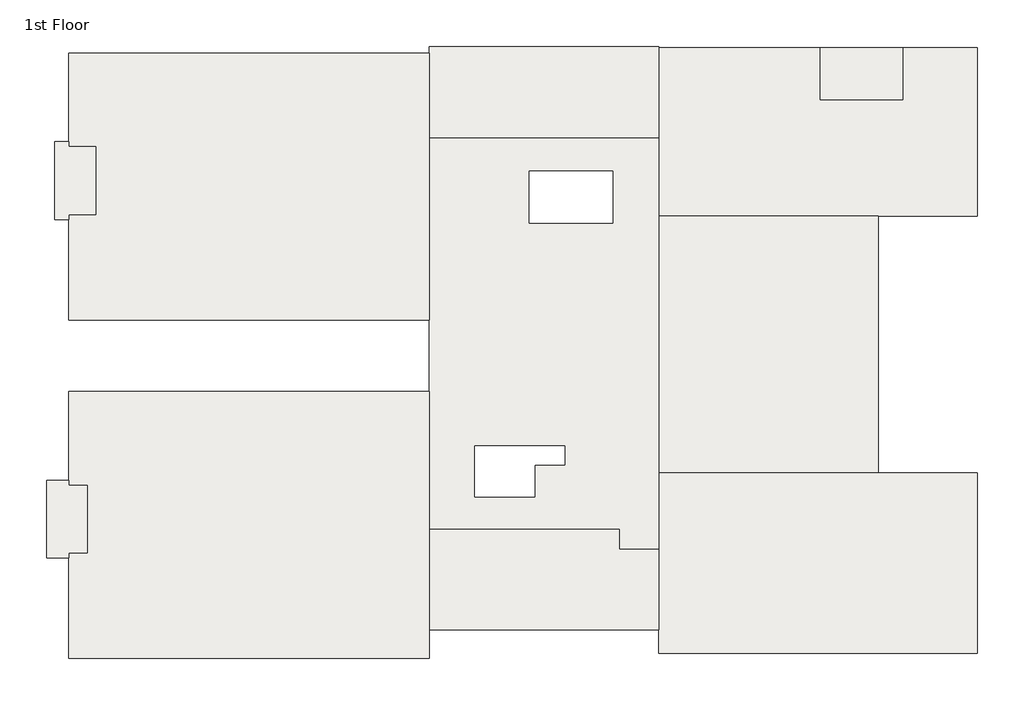
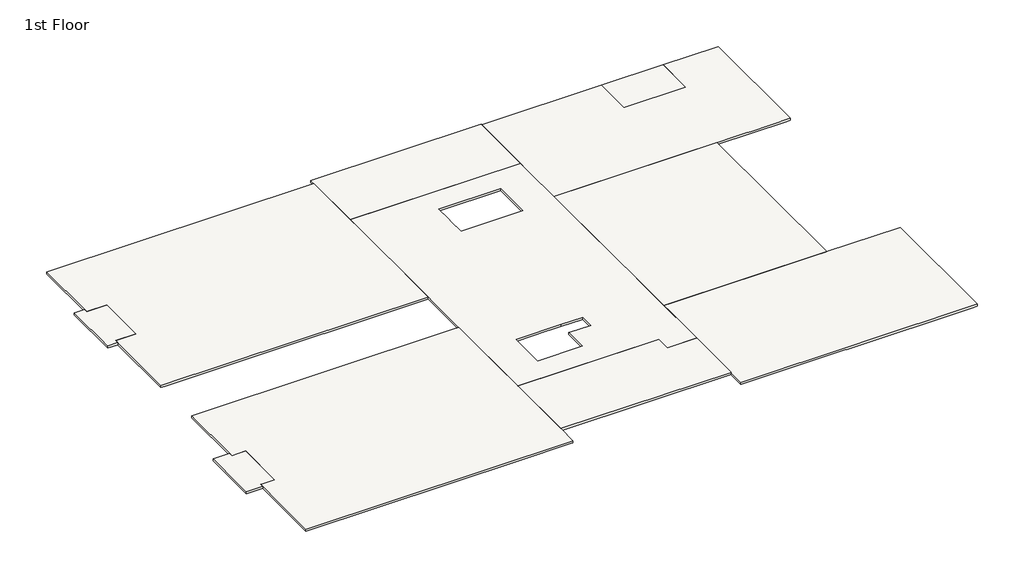
# One storey: 11 slabs.
"""IFC4 building model written with IfcOpenShell, lengths in millimetres."""

from ifc_helpers import new_model, si_unit, frame, origin, place, context, project, spatial, polyline, outline, extrude, faceted_brep, element, save

model = new_model("IFC4")

# Units and contexts
model_context = context("Model", 3, world=origin())
ifc_project = project(units=[si_unit("LENGTHUNIT", "METRE", prefix="MILLI")], contexts=[model_context])

# Site, building, storey
site = spatial("IfcSite", under=ifc_project)
building = spatial("IfcBuilding", under=site)
storey = spatial("IfcBuildingStorey", under=building, Name="1st Floor", Elevation=3200.4)

# Slabs
placement = place(None, origin())
element("IfcSlab", 1, at=placement, inside=storey, context=model_context, shape_type="Brep", body=[
    faceted_brep([(15770.2546318, 24595.834892, 3048.0), (15770.2546318, 4580.634892, 3048.0), (15770.2546318, 3564.634892, 3048.0), (13763.6546318, 3564.634892, 3048.0), (13763.6546318, 4580.634892, 3048.0), (12265.0546318, 4580.634892, 3048.0), (12087.2546318, 4580.634892, 3048.0), (9877.4546318, 4580.634892, 3048.0), (9699.6546318, 4580.634892, 3048.0), (7489.8546318, 4580.634892, 3048.0), (7312.0546318, 4580.634892, 3048.0), (4035.4546318, 4580.634892, 3048.0), (4035.4546318, 24595.834892, 3048.0), (7312.0546318, 24595.834892, 3048.0), (7489.8546318, 24595.834892, 3048.0), (9699.6546318, 24595.834892, 3048.0), (9877.4546318, 24595.834892, 3048.0), (12087.2546318, 24595.834892, 3048.0), (12265.0546318, 24595.834892, 3048.0), (9445.6546318, 8847.834892, 3048.0), (8836.0546318, 8847.834892, 3048.0), (8505.8546318, 8847.834892, 3048.0), (6372.2546318, 8847.834892, 3048.0), (6372.2546318, 6257.034892, 3048.0), (9445.6546318, 6257.034892, 3048.0), (9445.6546318, 7882.634892, 3048.0), (10969.6546318, 7882.634892, 3048.0), (10969.6546318, 8847.834892, 3048.0), (9166.2546318, 20252.434892, 3048.0), (13433.4546318, 20252.434892, 3048.0), (13433.4546318, 22919.434892, 3048.0), (9166.2546318, 22919.434892, 3048.0), (9166.2546318, 21751.034892, 3048.0), (9166.2546318, 21420.834892, 3048.0), (15770.2546318, 4580.634892, 3200.4), (15770.2546318, 24595.834892, 3200.4), (4035.4546318, 24595.834892, 3200.4), (4035.4546318, 11641.834892, 3200.4), (4035.4546318, 4580.634892, 3200.4), (13763.6546318, 4580.634892, 3200.4), (13763.6546318, 3564.634892, 3200.4), (15770.2546318, 3564.634892, 3200.4), (6372.2546318, 8847.834892, 3200.4), (9445.6546318, 8847.834892, 3200.4), (10969.6546318, 8847.834892, 3200.4), (10969.6546318, 7882.634892, 3200.4), (9445.6546318, 7882.634892, 3200.4), (9445.6546318, 6257.034892, 3200.4), (6372.2546318, 6257.034892, 3200.4), (13433.4546318, 20252.434892, 3200.4), (9166.2546318, 20252.434892, 3200.4), (9166.2546318, 21420.834892, 3200.4), (9166.2546318, 21751.034892, 3200.4), (9166.2546318, 22919.434892, 3200.4), (13433.4546318, 22919.434892, 3200.4)], [[[0, 1, 2, 3, 4, 5, 6, 7, 8, 9, 10, 11, 12, 13, 14, 15, 16, 17, 18], [19, 20, 21, 22, 23, 24, 25, 26, 27], [28, 29, 30, 31, 32, 33]], [[34, 35, 36, 37, 38, 39, 40, 41], [42, 43, 44, 45, 46, 47, 48], [49, 50, 51, 52, 53, 54]], [[1, 0, 35, 34]], [[11, 10, 9, 8, 7, 6, 5, 4, 39, 38]], [[12, 11, 38, 37, 36]], [[0, 18, 17, 16, 15, 14, 13, 12, 36, 35]], [[2, 1, 34, 41]], [[3, 2, 41, 40]], [[4, 3, 40, 39]], [[19, 43, 42, 22, 21, 20]], [[22, 42, 48, 23]], [[23, 48, 47, 24]], [[24, 47, 46, 25]], [[25, 46, 45, 26]], [[26, 45, 44, 27]], [[43, 19, 27, 44]], [[28, 50, 49, 29]], [[29, 49, 54, 30]], [[30, 54, 53, 31]], [[50, 28, 33, 32, 31, 53, 52, 51]]]),
])
element("IfcSlab", 2, at=placement, inside=storey, context=model_context, shape_type="Brep", body=[
    faceted_brep([(26997.0546318, 20608.034892, 3048.0), (26997.0546318, 7476.234892, 3048.0), (26743.0546318, 7476.234892, 3048.0), (15770.2546318, 7476.234892, 3048.0), (15770.2546318, 20608.034892, 3048.0), (19986.6546318, 20608.034892, 3048.0), (20240.6546318, 20608.034892, 3048.0), (22374.2546318, 20608.034892, 3048.0), (22628.2546318, 20608.034892, 3048.0), (26743.0546318, 20608.034892, 3048.0), (26997.0546318, 20608.034892, 3200.4), (15770.2546318, 20608.034892, 3200.4), (15770.2546318, 7476.234892, 3200.4), (26997.0546318, 7476.234892, 3200.4)], [[[0, 1, 2, 3, 4, 5, 6, 7, 8, 9]], [[10, 11, 12, 13]], [[1, 0, 10, 13]], [[3, 2, 1, 13, 12]], [[4, 3, 12, 11]], [[0, 9, 8, 7, 6, 5, 4, 11, 10]]]),
])
element("IfcSlab", 3, ObjectType="Cream Floor", at=placement, inside=storey, context=model_context, shape_type="Brep", body=[
    faceted_brep([(4035.4546318, 28964.634892, 3048.0), (4035.4546318, 24595.834892, 3048.0), (4035.4546318, 15299.434892, 3048.0), (428.6546318, 15299.434892, 3048.0), (-3101.9453682, 15299.434892, 3048.0), (-3279.7453682, 15299.434892, 3048.0), (-14138.2453682, 15299.434892, 3048.0), (-14392.2453682, 15299.434892, 3048.0), (-14392.2453682, 20430.234892, 3048.0), (-14392.2453682, 20684.234892, 3048.0), (-13007.9453682, 20684.234892, 3048.0), (-13007.9453682, 24164.034892, 3048.0), (-13490.5453682, 24164.034892, 3048.0), (-14392.2453682, 24164.034892, 3048.0), (-14392.2453682, 24418.034892, 3048.0), (-14392.2453682, 28710.634892, 3048.0), (-14392.2453682, 28964.634892, 3048.0), (3781.4546318, 28964.634892, 3048.0), (4035.4546318, 15299.434892, 3200.4), (4035.4546318, 24595.834892, 3200.4), (4035.4546318, 28964.634892, 3200.4), (-14392.2453682, 28964.634892, 3200.4), (-14392.2453682, 24418.034892, 3200.4), (-14392.2453682, 24164.034892, 3200.4), (-13007.9453682, 24164.034892, 3200.4), (-13007.9453682, 20684.234892, 3200.4), (-14392.2453682, 20684.234892, 3200.4), (-14392.2453682, 20430.234892, 3200.4), (-14392.2453682, 15299.434892, 3200.4)], [[[0, 1, 2, 3, 4, 5, 6, 7, 8, 9, 10, 11, 12, 13, 14, 15, 16, 17]], [[18, 19, 20, 21, 22, 23, 24, 25, 26, 27, 28]], [[2, 1, 0, 20, 19, 18]], [[7, 6, 5, 4, 3, 2, 18, 28]], [[7, 28, 27, 26, 9, 8]], [[10, 9, 26, 25]], [[11, 10, 25, 24]], [[13, 12, 11, 24, 23]], [[13, 23, 22, 21, 16, 15, 14]], [[0, 17, 16, 21, 20]]]),
])
element("IfcSlab", 4, ObjectType="Cream Floor", at=placement, inside=storey, context=model_context, shape_type="Brep", body=[
    faceted_brep([(4035.4546318, 11641.834892, 3048.0), (4035.4546318, 4580.634892, 3048.0), (4035.4546318, -550.165108, 3048.0), (4035.4546318, -1997.965108, 3048.0), (3781.4546318, -1997.965108, 3048.0), (403.2546318, -1997.965108, 3048.0), (-14392.2453682, -1997.965108, 3048.0), (-14392.2453682, -1743.965108, 3048.0), (-14392.2453682, 3132.834892, 3048.0), (-14392.2453682, 3386.834892, 3048.0), (-13439.7453682, 3386.834892, 3048.0), (-13439.7453682, 6841.234892, 3048.0), (-14138.2453682, 6841.234892, 3048.0), (-14392.2453682, 6841.234892, 3048.0), (-14392.2453682, 7095.234892, 3048.0), (-14392.2453682, 11387.834892, 3048.0), (-14392.2453682, 11641.834892, 3048.0), (3781.4546318, 11641.834892, 3048.0), (4035.4546318, 11641.834892, 3200.4), (3781.4546318, 11641.834892, 3200.4), (-14392.2453682, 11641.834892, 3200.4), (-14392.2453682, 7095.234892, 3200.4), (-14392.2453682, 6841.234892, 3200.4), (-13439.7453682, 6841.234892, 3200.4), (-13439.7453682, 3386.834892, 3200.4), (-14392.2453682, 3386.834892, 3200.4), (-14392.2453682, 3132.834892, 3200.4), (-14392.2453682, -1997.965108, 3200.4), (4035.4546318, -1997.965108, 3200.4), (4035.4546318, -550.165108, 3200.4), (4035.4546318, 4580.634892, 3200.4)], [[[0, 1, 2, 3, 4, 5, 6, 7, 8, 9, 10, 11, 12, 13, 14, 15, 16, 17]], [[18, 19, 20, 21, 22, 23, 24, 25, 26, 27, 28, 29, 30]], [[3, 2, 1, 0, 18, 30, 29, 28]], [[6, 5, 4, 3, 28, 27]], [[9, 8, 7, 6, 27, 26, 25]], [[10, 9, 25, 24]], [[11, 10, 24, 23]], [[13, 12, 11, 23, 22]], [[16, 15, 14, 13, 22, 21, 20]], [[0, 17, 16, 20, 19, 18]]]),
])
element("IfcSlab", 5, ObjectType="Cream Floor", at=placement, inside=storey, context=model_context, shape_type="Brep", body=[
    faceted_brep([(15770.2546318, -550.165108, 3048.0), (4035.4546318, -550.165108, 3048.0), (4035.4546318, -219.965108, 3048.0), (4035.4546318, 4326.634892, 3048.0), (4035.4546318, 4580.634892, 3048.0), (13509.6546318, 4580.634892, 3048.0), (13763.6546318, 4580.634892, 3048.0), (13763.6546318, 4326.634892, 3048.0), (13763.6546318, 3564.634892, 3048.0), (15770.2546318, 3564.634892, 3048.0), (15770.2546318, 3310.634892, 3048.0), (15770.2546318, -219.965108, 3048.0), (4035.4546318, -550.165108, 3200.4), (15770.2546318, -550.165108, 3200.4), (15770.2546318, 3564.634892, 3200.4), (13763.6546318, 3564.634892, 3200.4), (13763.6546318, 4580.634892, 3200.4), (4035.4546318, 4580.634892, 3200.4)], [[[0, 1, 2, 3, 4, 5, 6, 7, 8, 9, 10, 11]], [[12, 13, 14, 15, 16, 17]], [[1, 0, 13, 12]], [[4, 3, 2, 1, 12, 17]], [[6, 5, 4, 17, 16]], [[0, 11, 10, 9, 14, 13]], [[8, 7, 6, 16, 15]], [[9, 8, 15, 14]]]),
])
element("IfcSlab", 6, ObjectType="Cream Floor", at=placement, inside=storey, context=model_context, shape_type="Brep", body=[
    faceted_brep([(15770.2546318, 29294.834892, 3048.0), (15770.2546318, 28964.634892, 3048.0), (15770.2546318, 24595.834892, 3048.0), (13763.6546318, 24595.834892, 3048.0), (13509.6546318, 24595.834892, 3048.0), (6296.0546318, 24595.834892, 3048.0), (6042.0546318, 24595.834892, 3048.0), (4035.4546318, 24595.834892, 3048.0), (4035.4546318, 28964.634892, 3048.0), (4035.4546318, 29294.834892, 3048.0), (15770.2546318, 29294.834892, 3200.4), (4035.4546318, 29294.834892, 3200.4), (4035.4546318, 28964.634892, 3200.4), (4035.4546318, 24595.834892, 3200.4), (15770.2546318, 24595.834892, 3200.4)], [[[0, 1, 2, 3, 4, 5, 6, 7, 8, 9]], [[10, 11, 12, 13, 14]], [[2, 1, 0, 10, 14]], [[7, 6, 5, 4, 3, 2, 14, 13]], [[9, 8, 7, 13, 12, 11]], [[0, 9, 11, 10]]]),
])
element("IfcSlab", 7, ObjectType="Cream Floor", at=placement, inside=storey, context=model_context, shape_type="Brep", body=[
    faceted_brep([(15770.2546318, 20608.034892, 3048.0), (15770.2546318, 29244.034892, 3048.0), (16024.2546318, 29244.034892, 3048.0), (24025.2546318, 29244.034892, 3048.0), (24025.2546318, 28990.034892, 3048.0), (24025.2546318, 26551.634892, 3048.0), (28292.4546318, 26551.634892, 3048.0), (28292.4546318, 29244.034892, 3048.0), (28470.2546318, 29244.034892, 3048.0), (32077.0546318, 29244.034892, 3048.0), (32077.0546318, 28990.034892, 3048.0), (32077.0546318, 24570.434892, 3048.0), (32077.0546318, 20862.034892, 3048.0), (32077.0546318, 20608.034892, 3048.0), (31823.0546318, 20608.034892, 3048.0), (26997.0546318, 20608.034892, 3048.0), (16024.2546318, 20608.034892, 3048.0), (15770.2546318, 29244.034892, 3200.4), (15770.2546318, 20608.034892, 3200.4), (29079.8546318, 20608.034892, 3200.4), (29333.8546318, 20608.034892, 3200.4), (32077.0546318, 20608.034892, 3200.4), (32077.0546318, 29244.034892, 3200.4), (28292.4546318, 29244.034892, 3200.4), (28292.4546318, 26551.634892, 3200.4), (24025.2546318, 26551.634892, 3200.4), (24025.2546318, 29244.034892, 3200.4), (16024.2546318, 29244.034892, 3200.4)], [[[0, 1, 2, 3, 4, 5, 6, 7, 8, 9, 10, 11, 12, 13, 14, 15, 16]], [[17, 18, 19, 20, 21, 22, 23, 24, 25, 26, 27]], [[1, 0, 18, 17]], [[3, 2, 1, 17, 27, 26]], [[13, 12, 11, 10, 9, 22, 21]], [[0, 16, 15, 14, 13, 21, 20, 19, 18]], [[5, 4, 3, 26, 25]], [[6, 5, 25, 24]], [[7, 6, 24, 23]], [[9, 8, 7, 23, 22]]]),
])
element("IfcSlab", 8, ObjectType="Cream Floor", at=placement, inside=storey, context=model_context, shape_type="Brep", body=[
    faceted_brep([(32077.0546318, 7476.234892, 3048.0), (32077.0546318, 7222.234892, 3048.0), (32077.0546318, 3564.634892, 3048.0), (32077.0546318, 465.834892, 3048.0), (32077.0546318, -1743.965108, 3048.0), (31823.0546318, -1743.965108, 3048.0), (23085.4546318, -1743.965108, 3048.0), (22907.6546318, -1743.965108, 3048.0), (15770.2546318, -1743.965108, 3048.0), (15770.2546318, -1489.965108, 3048.0), (15770.2546318, 7476.234892, 3048.0), (16024.2546318, 7476.234892, 3048.0), (26997.0546318, 7476.234892, 3048.0), (28317.8546318, 7476.234892, 3048.0), (28571.8546318, 7476.234892, 3048.0), (32077.0546318, 7476.234892, 3200.4), (26997.0546318, 7476.234892, 3200.4), (15770.2546318, 7476.234892, 3200.4), (15770.2546318, -1743.965108, 3200.4), (32077.0546318, -1743.965108, 3200.4)], [[[0, 1, 2, 3, 4, 5, 6, 7, 8, 9, 10, 11, 12, 13, 14]], [[15, 16, 17, 18, 19]], [[4, 3, 2, 1, 0, 15, 19]], [[8, 7, 6, 5, 4, 19, 18]], [[10, 9, 8, 18, 17]], [[0, 14, 13, 12, 11, 10, 17, 16, 15]]]),
])
element("IfcSlab", 9, ObjectType="Deck 1", at=placement, inside=storey, context=model_context, shape_type="SweptSolid", body=[
    extrude(outline(polyline([(-14392.2453682, 24418.034892), (-14392.2453682, 24164.034892), (-13007.9453682, 24164.034892), (-13007.9453682, 20684.234892), (-14392.2453682, 20684.234892), (-14392.2453682, 20430.234892), (-15090.7453682, 20430.234892), (-15090.7453682, 24418.034892), (-14392.2453682, 24418.034892)])), frame((0.0, 0.0, 3048.0), z_axis=(0.0, 0.0, 1.0), x_axis=(1.0, 0.0, 0.0)), (0.0, 0.0, 1.0), 152.4),
])
element("IfcSlab", 10, ObjectType="Deck 1", at=placement, inside=storey, context=model_context, shape_type="SweptSolid", body=[
    extrude(outline(polyline([(-14392.2453682, 7095.234892), (-14392.2453682, 6841.234892), (-13439.7453682, 6841.234892), (-13439.7453682, 3386.834892), (-14392.2453682, 3386.834892), (-14392.2453682, 3132.834892), (-15522.5453682, 3132.834892), (-15522.5453682, 7095.234892), (-14392.2453682, 7095.234892)])), frame((0.0, 0.0, 3048.0), z_axis=(0.0, 0.0, 1.0), x_axis=(1.0, 0.0, 0.0)), (0.0, 0.0, 1.0), 152.4),
])
element("IfcSlab", 11, ObjectType="Deck 1", at=placement, inside=storey, context=model_context, shape_type="SweptSolid", body=[
    extrude(outline(polyline([(28292.4546318, 29244.034892), (28292.4546318, 26551.634892), (24025.2546318, 26551.634892), (24025.2546318, 29244.034892), (28292.4546318, 29244.034892)])), frame((0.0, 0.0, 3048.0), z_axis=(0.0, 0.0, 1.0), x_axis=(1.0, 0.0, 0.0)), (0.0, 0.0, 1.0), 152.4),
])

save(model, "model.ifc")

# Revit data of these elements
# Type
#   Assembly Code = "B1010"
#   Function = 0
#   Layers, outside or top first: 0' - 6" "0 reception tile" (function 1)
# Type "Cream Floor"
#   Assembly Code = "B1010"
#   Function = 0
#   Layers, outside or top first: 0' - 6" "0 cream Floor" (function 1)
# Type "Deck 1"
#   Assembly Code = "B1010"
#   Function = 0
#   Layers, outside or top first: 0' - 6" "0 deck(1)" (function 1)
# Element 1 (IfcSlab)
#   Height Offset From Level = 0' - 0"
#   Phase Created = New Construction
#   Materials on its faces: "0 reception tile"
# Element 2 (IfcSlab)
#   Height Offset From Level = 0' - 0"
#   Phase Created = New Construction
#   Materials on its faces: "0 reception tile", "0 olive green"
# Elements 3, 4, 5, 6 (IfcSlab, "Cream Floor")
#   Height Offset From Level = 0' - 0"
#   Phase Created = New Construction
#   Materials on its faces: "0 cream Floor", "0 olive green"
# Element 7 (IfcSlab, "Cream Floor")
#   built-in parameter 1001955 = 3.14159 (stored number, unit not read)
#   Height Offset From Level = 0' - 0"
#   Phase Created = New Construction
#   Materials on its faces: "0 cream Floor", "0 olive green"
# Element 8 (IfcSlab, "Cream Floor")
#   Height Offset From Level = 0' - 0"
#   Phase Created = New Construction
#   Materials on its faces: "0 olive green", "0 cream Floor"
# Elements 9, 10, 11 (IfcSlab, "Deck 1")
#   Height Offset From Level = 0' - 0"
#   Phase Created = New Construction
#   Materials on its faces: "0 deck(1)", "0 olive green"
# Materials
#   "0 reception tile": class "Generic", colour RGB 120 120 120, transparency 0, Cost = 0
#   "0 cream Floor": class "Generic", colour RGB 120 120 120, transparency 0, Cost = 0
#   "0 deck(1)": class "Generic", colour RGB 120 120 120, transparency 0, Cost = 0
#   "0 olive green": class "Generic", colour RGB 120 120 120, transparency 0, Cost = 0
